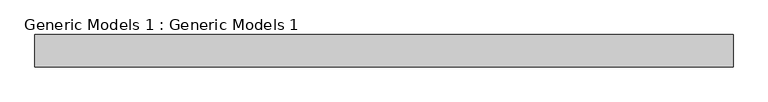
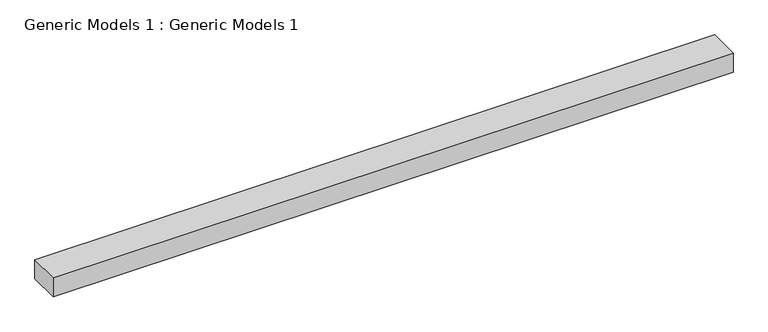
"""IFC4 building model written with IfcOpenShell, lengths in millimetres: proxy geometry, Generic Models 1 : Generic Models 1."""

from ifc_helpers import new_model, si_unit, frame, origin, place, context, project, spatial, polyline, outline, extrude, source, transform, mapped, element, save


def generic_models_1_generic_models_1_77739e1a(model_context):
    return source(origin(), model_context, "Body", "SweptSolid", [
        extrude(outline(polyline([(-7701.088074, -21418.2982388), (-7701.088074, -20921.9985361), (2992.311926, -20921.9985361), (2992.311926, -21418.2982388), (-7701.088074, -21418.2982388)])), frame((0.0, 0.0, 36040.1219411), z_axis=(0.0, 0.0, 1.0), x_axis=(1.0, 0.0, 0.0)), (0.0, 0.0, 1.0), 318.5447205),
    ])


if __name__ == "__main__":
    model = new_model("IFC4")
    model_context = context("Model", 3, world=origin())
    ifc_project = project(units=[si_unit("LENGTHUNIT", "METRE", prefix="MILLI")], contexts=[model_context])
    site = spatial("IfcSite", under=ifc_project)
    building = spatial("IfcBuilding", under=site)
    placement = place(None, origin())
    generic_models_1_generic_models_1_shape = generic_models_1_generic_models_1_77739e1a(model_context)
    element("IfcBuildingElementProxy", 1, Name="Generic Models 1 : Generic Models 1", ObjectType="Generic Models 1 : Generic Models 1", at=placement, inside=building, context=model_context, shape_type="MappedRepresentation", body=[
        mapped(generic_models_1_generic_models_1_shape, transform((0.0, 0.0, 0.0), x_axis=(1.0, 0.0, 0.0), y_axis=(0.0, 1.0, 0.0), z_axis=(0.0, 0.0, 1.0))),
    ])
    save(model, "model.ifc")
